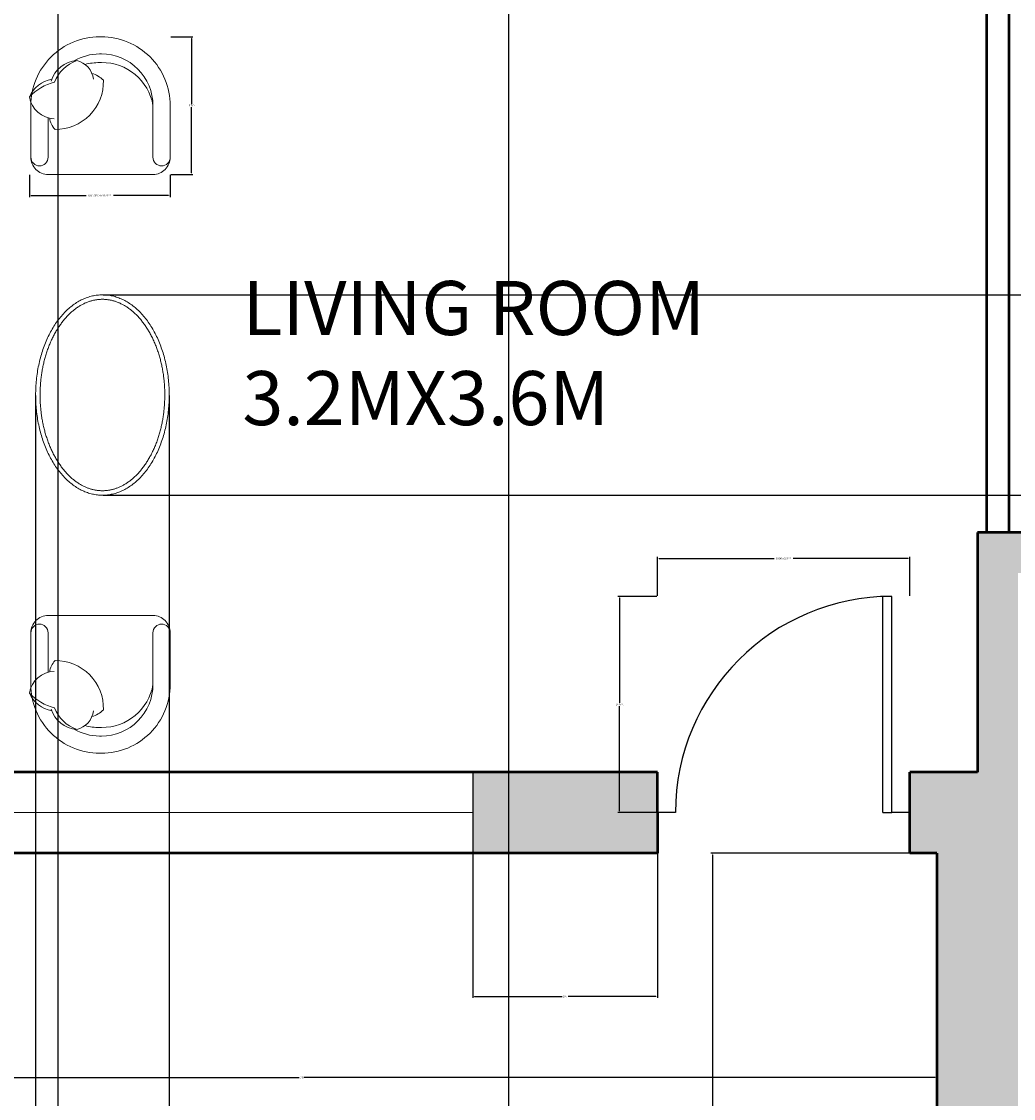
# Model space of a CAD drawing. Units: inches. Extents: x 3 to 380, y -485 to 60.
# Tile 3 of 8: x 67 to 177, y -390 to -270. Entities that reach past the tile are written whole.
import ezdxf

# ---------------------------------------------------------------- set-up
doc = ezdxf.new("R2010")
doc.units = ezdxf.units.IN
doc.header["$MEASUREMENT"] = 0
for name, color, linetype, lineweight in [('A-ANNO-DIMS', 2, 'Continuous', 18), ('A-AREA-IDEN', 7, 'Continuous', 25), ('A-DOOR', 3, 'Continuous', 25), ('A-FURN', 8, 'Continuous', 18), ('A-GLAZ', 4, 'Continuous', 18), ('A-WALL', 7, 'Continuous', 50), ('A-WALL-PATT', 252, 'Continuous', 13)]:
    doc.layers.add(name, color=color, linetype=linetype, lineweight=lineweight)
doc.styles.get("Standard").update_dxf_attribs({"font": 'arial.ttf'})
doc.dimstyles.get("Standard").update_dxf_attribs({"dimtxt": 0.18, "dimasz": 0.18, "dimexe": 0.18, "dimexo": 0.0625, "dimgap": 0.09, "dimtad": 0, "dimtih": 1, "dimtoh": 1, "dimdec": 0, "dimzin": 0, "dimdsep": 46, "dimlunit": 3, "dimtxsty": 'Standard', "dimcen": 0.09, "dimadec": 0, "dimazin": 0, "dimtfac": 1, "dimtdec": 0, "dimtofl": 0, "dimtmove": 0, "dimatfit": 3, "dimfxl": 1, "dimtolj": 1, "dimtzin": 0, "dimarcsym": 0})

# ---------------------------------------------------------------- blocks, each defined once
blk = doc.blocks.new('LOUNGE-CHAIR')
at = {"ltscale": 0.03}
blk.add_lwpolyline([(7.89, 0), (13.71, 0, 0.414214), (15.62, 1.91), (15.62, 7.64, 0.414214), (7.98, 15.28), (7.89, 15.28), (7.79, 15.28, 0.414214), (0.16, 7.64), (0.16, 1.91, 0.414214), (2.07, 0), (7.89, 0)], format="xyb", dxfattribs=at)
for points in [[(4.95, 12.61, -0.130591), (7.79, 13.37), (7.89, 13.37)], [(13.71, 7.64, 0.414214), (7.98, 13.37), (7.89, 13.37)], [(0, 8.6, -0.14773), (2.79, 10.24, -0.213343), (5.25, 12.65, -0.178662)], [(2.4, 10.37, -0.306663), (5.25, 12.65, -0.30633), (7.11, 10.57, 0.872847)], [(6.17, 12.21, -0.072384), (7.79, 12.41), (7.89, 12.41)], [(13.71, 7.64, 0.372719), (7.98, 12.41), (7.89, 12.41)], [(2.25, 6.25, 0.165541), (2.84, 4.99, 0.425989), (8.21, 10.46, 0.121523), (6.93, 11.21, -7.115464)], [(2.74, 6.19, -0.356772), (0, 8.6, -0.249542), (2.48, 10.58, 9.61688)], [(13.71, 7.64), (13.71, 1.91, 0.414214), (14.67, 0.95), (14.67, 0.95, 0.414214), (15.62, 1.91)], [(2.07, 6.3), (2.07, 1.91, -0.414214), (1.11, 0.95), (1.11, 0.95, -0.414214), (0.16, 1.91)]]:
    blk.add_lwpolyline(points, format="xyb")
blk = doc.blocks.new('WIN-60X9-SPLIT-JAMB')
for p, q in [((60, 9), (0, 9)), ((0, 9), (0, 0)), ((60, 4.5), (60, 9)), ((0, 4.5), (60, 4.5)), ((60, 4.5), (60, 0)), ((0, 0), (60, 0))]:
    blk.add_line(p, q)
blk = doc.blocks.new('DOOR-SWING-24')
for p, q in [((25, 0), (25, 24)), ((26, 0), (26, 24)), ((2, 0), (0, 0)), ((25, 0), (26, 0)), ((28, 0), (26, 0))]:
    blk.add_line(p, q)
blk.add_arc((26, 0), 24, 90, 180)
blk = doc.blocks.new('*D23')
at = {"layer": 'A-ANNO-DIMS', "color": 0, "lineweight": -2, "transparency": 16777216}
for p, q in [((137.84, -333.87), (137.84, -329.55)), ((138.02, -329.73), (150.79, -329.73)), ((165.66, -329.73), (152.89, -329.73)), ((165.84, -333.87), (165.84, -329.55))]:
    blk.add_line(p, q, dxfattribs=at)
at = {"layer": 'A-ANNO-DIMS', "color": 0, "transparency": 16777216}
for points in [[(138.02, -329.7), (138.02, -329.76), (137.84, -329.73)], [(165.66, -329.7), (165.66, -329.76), (165.84, -329.73)]]:
    blk.add_solid(points, dxfattribs=at)
at = {"layer": 'Defpoints', "color": 0, "transparency": 16777216}
for p in [(165.84, -329.73), (137.84, -333.93), (165.84, -333.93)]:
    blk.add_point(p, dxfattribs=at)
at = {"layer": 'A-ANNO-DIMS', "color": 0, "transparency": 16777216, "insert": (151.84, -329.73), "char_height": 0.18, "attachment_point": 5}
blk.add_mtext('\\A1;DOOR A 28 TYP.', dxfattribs=at)
blk = doc.blocks.new('*D24')
at = {"layer": 'A-ANNO-DIMS', "color": 0, "lineweight": -2, "transparency": 16777216}
for p, q in [((137.78, -333.93), (133.46, -333.93)), ((133.64, -334.11), (133.64, -345.75)), ((133.64, -357.75), (133.64, -346.11)), ((137.78, -357.93), (133.46, -357.93))]:
    blk.add_line(p, q, dxfattribs=at)
at = {"layer": 'A-ANNO-DIMS', "color": 0, "transparency": 16777216}
for points in [[(133.61, -334.11), (133.67, -334.11), (133.64, -333.93)], [(133.61, -357.75), (133.67, -357.75), (133.64, -357.93)]]:
    blk.add_solid(points, dxfattribs=at)
at = {"layer": 'Defpoints', "color": 0, "transparency": 16777216}
for p in [(133.64, -333.93), (137.84, -333.93), (137.84, -357.93)]:
    blk.add_point(p, dxfattribs=at)
at = {"layer": 'A-ANNO-DIMS', "color": 0, "transparency": 16777216, "insert": (133.64, -345.93), "char_height": 0.18, "attachment_point": 5}
blk.add_mtext('\\A1;24 TYP.', dxfattribs=at)
blk = doc.blocks.new('*D39')
at = {"layer": 'A-ANNO-DIMS', "color": 0, "lineweight": -2, "transparency": 16777216}
for p, q in [((68.15, -287.16), (68.15, -289.62)), ((83.78, -287.16), (83.78, -289.62)), ((68.33, -289.44), (74.45, -289.44)), ((83.6, -289.44), (77.48, -289.44))]:
    blk.add_line(p, q, dxfattribs=at)
at = {"layer": 'A-ANNO-DIMS', "color": 0, "transparency": 16777216}
for points in [[(68.33, -289.41), (68.33, -289.47), (68.15, -289.44)], [(83.6, -289.41), (83.6, -289.47), (83.78, -289.44)]]:
    blk.add_solid(points, dxfattribs=at)
at = {"layer": 'Defpoints', "color": 0, "transparency": 16777216}
for p in [(68.15, -287.1), (83.78, -287.1), (83.78, -289.44)]:
    blk.add_point(p, dxfattribs=at)
at = {"layer": 'A-ANNO-DIMS', "color": 0, "transparency": 16777216, "insert": (75.96, -289.44), "char_height": 0.18, "attachment_point": 5}
blk.add_mtext('\\A1;LOUNGE CHAIR 16 TYP.', dxfattribs=at)
blk = doc.blocks.new('*D40')
at = {"layer": 'A-ANNO-DIMS', "color": 0, "lineweight": -2, "transparency": 16777216}
for p, q in [((83.84, -271.82), (86.3, -271.82)), ((86.12, -272), (86.12, -279.28)), ((86.12, -286.92), (86.12, -279.64)), ((83.84, -287.1), (86.3, -287.1))]:
    blk.add_line(p, q, dxfattribs=at)
at = {"layer": 'A-ANNO-DIMS', "color": 0, "transparency": 16777216}
for points in [[(86.09, -272), (86.15, -272), (86.12, -271.82)], [(86.09, -286.92), (86.15, -286.92), (86.12, -287.1)]]:
    blk.add_solid(points, dxfattribs=at)
at = {"layer": 'Defpoints', "color": 0, "transparency": 16777216}
for p in [(83.78, -271.82), (86.12, -271.82), (83.78, -287.1)]:
    blk.add_point(p, dxfattribs=at)
at = {"layer": 'A-ANNO-DIMS', "color": 0, "transparency": 16777216, "insert": (86.12, -279.46), "char_height": 0.18, "attachment_point": 5}
blk.add_mtext('\\A1;15 TYP.', dxfattribs=at)
blk = doc.blocks.new('*D51')
at = {"layer": 'A-ANNO-DIMS', "color": 0, "lineweight": -2, "transparency": 16777216}
for p, q in [((151.9, 34.66), (379.92, 34.66)), ((379.74, 34.48), (379.74, -212.65)), ((379.74, -460.16), (379.74, -213.02)), ((354.9, -460.34), (379.92, -460.34))]:
    blk.add_line(p, q, dxfattribs=at)
at = {"layer": 'A-ANNO-DIMS', "color": 0, "transparency": 16777216}
for points in [[(379.71, 34.48), (379.77, 34.48), (379.74, 34.66)], [(379.71, -460.16), (379.77, -460.16), (379.74, -460.34)]]:
    blk.add_solid(points, dxfattribs=at)
at = {"layer": 'Defpoints', "color": 0, "transparency": 16777216}
for p in [(151.84, 34.66), (354.84, -460.34), (379.74, -460.34)]:
    blk.add_point(p, dxfattribs=at)
at = {"layer": 'A-ANNO-DIMS', "color": 0, "transparency": 16777216, "insert": (379.74, -212.84), "char_height": 0.18, "attachment_point": 5}
blk.add_mtext('\\A1;495', dxfattribs=at)
blk = doc.blocks.new('*D52')
at = {"layer": 'A-ANNO-DIMS', "color": 0, "lineweight": -2, "transparency": 16777216}
for p, q in [((27.84, -362.49), (27.84, -387.51)), ((168.84, -362.49), (168.84, -387.51)), ((28.02, -387.33), (98.08, -387.33)), ((168.66, -387.33), (98.6, -387.33))]:
    blk.add_line(p, q, dxfattribs=at)
at = {"layer": 'A-ANNO-DIMS', "color": 0, "transparency": 16777216}
for points in [[(28.02, -387.3), (28.02, -387.36), (27.84, -387.33)], [(168.66, -387.3), (168.66, -387.36), (168.84, -387.33)]]:
    blk.add_solid(points, dxfattribs=at)
at = {"layer": 'Defpoints', "color": 0, "transparency": 16777216}
for p in [(27.84, -362.43), (168.84, -362.43), (27.84, -387.33)]:
    blk.add_point(p, dxfattribs=at)
at = {"layer": 'A-ANNO-DIMS', "color": 0, "transparency": 16777216, "insert": (98.34, -387.33), "char_height": 0.18, "attachment_point": 5}
blk.add_mtext('\\A1;141', dxfattribs=at)
blk = doc.blocks.new('*D56')
at = {"layer": 'A-ANNO-DIMS', "color": 0, "lineweight": -2, "transparency": 16777216}
for p, q in [((168.78, -362.43), (143.76, -362.43)), ((143.94, -362.61), (143.94, -411.2)), ((143.94, -460.16), (143.94, -411.56)), ((168.78, -460.34), (143.76, -460.34))]:
    blk.add_line(p, q, dxfattribs=at)
at = {"layer": 'A-ANNO-DIMS', "color": 0, "transparency": 16777216}
for points in [[(143.91, -362.61), (143.97, -362.61), (143.94, -362.43)], [(143.91, -460.16), (143.97, -460.16), (143.94, -460.34)]]:
    blk.add_solid(points, dxfattribs=at)
at = {"layer": 'Defpoints', "color": 0, "transparency": 16777216}
for p in [(143.94, -362.43), (168.84, -362.43), (168.84, -460.34)]:
    blk.add_point(p, dxfattribs=at)
at = {"layer": 'A-ANNO-DIMS', "color": 0, "transparency": 16777216, "insert": (143.94, -411.38), "char_height": 0.18, "attachment_point": 5}
blk.add_mtext('\\A1;97.9', dxfattribs=at)
blk = doc.blocks.new('*D82')
at = {"layer": 'A-ANNO-DIMS', "color": 0, "lineweight": -2, "transparency": 16777216}
for p, q in [((117.34, -353.49), (117.34, -378.51)), ((137.84, -353.49), (137.84, -378.51)), ((117.52, -378.33), (127.26, -378.33)), ((137.66, -378.33), (127.92, -378.33))]:
    blk.add_line(p, q, dxfattribs=at)
at = {"layer": 'A-ANNO-DIMS', "color": 0, "transparency": 16777216}
for points in [[(117.52, -378.3), (117.52, -378.36), (117.34, -378.33)], [(137.66, -378.3), (137.66, -378.36), (137.84, -378.33)]]:
    blk.add_solid(points, dxfattribs=at)
at = {"layer": 'Defpoints', "color": 0, "transparency": 16777216}
for p in [(117.34, -353.43), (137.84, -353.43), (117.34, -378.33)]:
    blk.add_point(p, dxfattribs=at)
at = {"layer": 'A-ANNO-DIMS', "color": 0, "transparency": 16777216, "insert": (127.59, -378.33), "char_height": 0.18, "attachment_point": 5}
blk.add_mtext('\\A1;20.5', dxfattribs=at)
blk = doc.blocks.new('*D93')
at = {"layer": 'A-ANNO-DIMS', "color": 0, "lineweight": -2, "transparency": 16777216}
for p, q in [((71.32, -23.85), (71.32, -485.42)), ((121.32, -23.85), (121.32, -485.42)), ((71.5, -485.24), (95.92, -485.24)), ((121.14, -485.24), (96.72, -485.24))]:
    blk.add_line(p, q, dxfattribs=at)
at = {"layer": 'A-ANNO-DIMS', "color": 0, "transparency": 16777216}
for points in [[(71.5, -485.21), (71.5, -485.27), (71.32, -485.24)], [(121.14, -485.21), (121.14, -485.27), (121.32, -485.24)]]:
    blk.add_solid(points, dxfattribs=at)
at = {"layer": 'Defpoints', "color": 0, "transparency": 16777216}
for p in [(71.32, -23.79), (121.32, -23.79), (71.32, -485.24)]:
    blk.add_point(p, dxfattribs=at)
at = {"layer": 'A-ANNO-DIMS', "color": 0, "transparency": 16777216, "insert": (96.32, -485.24), "char_height": 0.18, "attachment_point": 5}
blk.add_mtext('\\A1;49.99', dxfattribs=at)
blk = doc.blocks.new('*D99')
at = {"layer": 'A-ANNO-DIMS', "color": 0, "lineweight": -2, "transparency": 16777216}
for p, q in [((76.32, -300.46), (379.92, -300.46)), ((379.74, -300.64), (379.74, -311.4)), ((379.74, -322.52), (379.74, -311.76)), ((76.32, -322.7), (379.92, -322.7))]:
    blk.add_line(p, q, dxfattribs=at)
at = {"layer": 'A-ANNO-DIMS', "color": 0, "transparency": 16777216}
for points in [[(379.71, -300.64), (379.77, -300.64), (379.74, -300.46)], [(379.71, -322.52), (379.77, -322.52), (379.74, -322.7)]]:
    blk.add_solid(points, dxfattribs=at)
at = {"layer": 'Defpoints', "color": 0, "transparency": 16777216}
for p in [(76.25, -300.46), (76.25, -322.7), (379.74, -322.7)]:
    blk.add_point(p, dxfattribs=at)
at = {"layer": 'A-ANNO-DIMS', "color": 0, "transparency": 16777216, "insert": (379.74, -311.58), "char_height": 0.18, "attachment_point": 5}
blk.add_mtext('\\A1;22.236', dxfattribs=at)
blk = doc.blocks.new('*D100')
at = {"layer": 'A-ANNO-DIMS', "color": 0, "lineweight": -2, "transparency": 16777216}
for p, q in [((68.84, -311.64), (68.84, -485.42)), ((83.67, -311.64), (83.67, -485.42)), ((69.02, -485.24), (75.8, -485.24)), ((83.49, -485.24), (76.71, -485.24))]:
    blk.add_line(p, q, dxfattribs=at)
at = {"layer": 'A-ANNO-DIMS', "color": 0, "transparency": 16777216}
for points in [[(69.02, -485.21), (69.02, -485.27), (68.84, -485.24)], [(83.49, -485.21), (83.49, -485.27), (83.67, -485.24)]]:
    blk.add_solid(points, dxfattribs=at)
at = {"layer": 'Defpoints', "color": 0, "transparency": 16777216}
for p in [(68.84, -311.58), (83.67, -311.58), (83.67, -485.24)]:
    blk.add_point(p, dxfattribs=at)
at = {"layer": 'A-ANNO-DIMS', "color": 0, "transparency": 16777216, "insert": (76.25, -485.24), "char_height": 0.18, "attachment_point": 5}
blk.add_mtext('\\A1;14.824', dxfattribs=at)

msp = doc.modelspace()

# ---------------------------------------------------------------- hatches: boundary and pattern name
at = {"layer": 'A-WALL-PATT'}
h = msp.add_hatch(color=256, dxfattribs=at)
h.dxf.hatch_style = 1
h.paths.add_polyline_path([(36.8404, 6.1643), (51.3404, 6.1643), (51.3404, 15.1643), (27.8404, 15.1643), (27.8404, -143.6318), (36.8404, -143.6318)])
h.paths.add_polyline_path([(125.8404, 10.6643), (125.8404, 15.1643), (111.3404, 15.1643), (111.3404, 6.1643), (125.8404, 6.1643)])
h.paths.add_polyline_path([(170.6358, 15.1643), (153.8404, 15.1643), (153.8404, 6.1643), (156.8404, 6.1643), (156.8404, -82.3357), (173.3404, -82.3357), (173.3404, -130.3357), (177.8404, -130.3357), (180.8404, -130.3357), (180.8404, -125.8357), (177.8404, -125.8357), (177.8404, -82.3357), (201.8404, -82.3357), (201.8404, -38.0857), (197.3404, -38.0857), (197.3404, -77.8357), (161.3404, -77.8357), (161.3404, 6.1643), (170.6358, 6.1643)])
h.paths.add_polyline_path([(241.3739, 15.1643), (194.6358, 15.1643), (194.6358, 6.1643), (241.3739, 6.1643)])
h.paths.add_polyline_path([(201.8404, 6.1643), (197.3404, 6.1643), (197.3404, -12.1977), (201.8404, -12.1977)], flags=17)
h.paths.add_polyline_path([(354.8404, 15.1643), (301.3739, 15.1643), (301.3739, 6.1643), (345.8404, 6.1643), (345.8404, -34.0336), (354.8404, -34.0336)])
h.paths.add_polyline_path([(354.8404, -94.0336), (345.8404, -94.0336), (345.8404, -159.3738), (354.8404, -159.3738)])
h.paths.add_polyline_path([(345.8404, -125.8357), (209.3404, -125.8357), (209.3404, -205.8357), (211.5904, -205.8357), (213.8404, -205.8357), (213.8404, -130.3357), (345.8404, -130.3357)])
h.paths.add_polyline_path([(36.8404, -203.6318), (27.8404, -203.6318), (27.8404, -270.1269), (36.8404, -270.1269)])
h.paths.add_polyline_path([(36.8404, -330.1269), (27.8404, -330.1269), (27.8404, -362.428), (57.3404, -362.428), (57.3404, -353.428), (36.8404, -353.428)])
h.paths.add_polyline_path([(177.8404, -331.3357), (180.8404, -331.3357), (180.8404, -326.8357), (173.3404, -326.8357), (173.3404, -353.428), (165.8404, -353.428), (165.8404, -362.428), (168.8404, -362.428), (168.8404, -451.3357), (168.8404, -460.3357), (231.8404, -460.3357), (231.8404, -451.3357), (177.8404, -451.3357)])
h.paths.add_polyline_path([(354.8404, -305.1003), (345.8404, -305.1003), (345.8404, -363.2829), (354.8404, -363.2829)])
h.paths.add_polyline_path([(345.8404, -326.8357), (213.8404, -326.8357), (213.8404, -312.8357), (211.5904, -312.8357), (209.3404, -312.8357), (209.3404, -331.3357), (345.8404, -331.3357)])
h.paths.add_polyline_path([(345.8404, -262.3357), (237.8404, -262.3357), (237.8404, -233.8357), (209.3404, -233.8357), (209.3404, -284.8357), (213.8404, -284.8357), (213.8404, -238.3357), (233.3404, -238.3357), (233.3404, -266.8357), (345.8404, -266.8357)])
h.paths.add_polyline_path([(354.8404, -219.3738), (345.8404, -219.3738), (345.8404, -281.1003), (354.8404, -281.1003)])
h = msp.add_hatch(color=256, dxfattribs=at)
h.dxf.hatch_style = 1
h.paths.add_polyline_path([(137.8404, -353.428), (117.3404, -353.428), (117.3404, -357.928), (117.3404, -362.428), (137.8404, -362.428), (137.8404, -357.928)])

# ---------------------------------------------------------------- linework, layer by layer
at = {"layer": 'A-FURN', "ltscale": 0.03}
msp.add_polyline3d([(76.2547, -300.4625, 0), (76.1145, -300.4645, 0), (75.9742, -300.4705, 0), (75.8341, -300.4804, 0), (75.6942, -300.4943, 0), (75.5544, -300.5122, 0), (75.4149, -300.5341, 0), (75.2757, -300.5599, 0), (75.1368, -300.5897, 0), (74.9983, -300.6234, 0), (74.8603, -300.661, 0), (74.7228, -300.7026, 0), (74.5859, -300.748, 0), (74.4495, -300.7973, 0), (74.3138, -300.8505, 0), (74.1787, -300.9075, 0), (74.0445, -300.9683, 0), (73.911, -301.033, 0), (73.7783, -301.1014, 0), (73.6466, -301.1736, 0), (73.5157, -301.2495, 0), (73.3859, -301.3291, 0), (73.2571, -301.4123, 0), (73.1293, -301.4992, 0), (73.0027, -301.5898, 0), (72.8772, -301.6839, 0), (72.753, -301.7815, 0), (72.63, -301.8827, 0), (72.5083, -301.9873, 0), (72.3879, -302.0954, 0), (72.269, -302.2068, 0), (72.1514, -302.3216, 0), (72.0353, -302.4398, 0), (71.9208, -302.5612, 0), (71.8078, -302.6858, 0), (71.6963, -302.8137, 0), (71.5865, -302.9446, 0), (71.4784, -303.0787, 0), (71.372, -303.2158, 0), (71.2674, -303.3559, 0), (71.1645, -303.4989, 0), (71.0635, -303.6449, 0), (70.9643, -303.7936, 0), (70.867, -303.9452, 0), (70.7716, -304.0995, 0), (70.6782, -304.2565, 0), (70.5868, -304.4161, 0), (70.4974, -304.5783, 0), (70.4101, -304.743, 0), (70.3249, -304.9101, 0), (70.2418, -305.0796, 0), (70.1609, -305.2515, 0), (70.0821, -305.4256, 0), (70.0056, -305.6019, 0), (69.9313, -305.7804, 0), (69.8592, -305.9609, 0), (69.7895, -306.1434, 0), (69.722, -306.3279, 0), (69.6569, -306.5143, 0), (69.5942, -306.7025, 0), (69.5339, -306.8925, 0), (69.4759, -307.0841, 0), (69.4204, -307.2773, 0), (69.3673, -307.4721, 0), (69.3167, -307.6683, 0), (69.2686, -307.866, 0), (69.223, -308.0649, 0), (69.1799, -308.2652, 0), (69.1393, -308.4666, 0), (69.1013, -308.6691, 0), (69.0659, -308.8727, 0), (69.033, -309.0773, 0), (69.0027, -309.2827, 0), (68.975, -309.489, 0), (68.9499, -309.696, 0), (68.9275, -309.9037, 0), (68.9076, -310.112, 0), (68.8904, -310.3208, 0), (68.8759, -310.5301, 0), (68.8639, -310.7397, 0), (68.8546, -310.9496, 0), (68.848, -311.1598, 0), (68.844, -311.3701, 0), (68.8427, -311.5805, 0), (68.844, -311.7909, 0), (68.848, -312.0013, 0), (68.8546, -312.2114, 0), (68.8639, -312.4214, 0), (68.8759, -312.631, 0), (68.8904, -312.8403, 0), (68.9076, -313.0491, 0), (68.9275, -313.2574, 0), (68.9499, -313.4651, 0), (68.975, -313.6721, 0), (69.0027, -313.8784, 0), (69.033, -314.0838, 0), (69.0659, -314.2884, 0), (69.1013, -314.492, 0), (69.1393, -314.6945, 0), (69.1799, -314.8959, 0), (69.223, -315.0962, 0), (69.2686, -315.2951, 0), (69.3167, -315.4928, 0), (69.3673, -315.689, 0), (69.4204, -315.8838, 0), (69.4759, -316.077, 0), (69.5339, -316.2686, 0), (69.5942, -316.4586, 0), (69.6569, -316.6468, 0), (69.722, -316.8331, 0), (69.7895, -317.0176, 0), (69.8592, -317.2002, 0), (69.9313, -317.3807, 0), (70.0056, -317.5592, 0), (70.0821, -317.7355, 0), (70.1609, -317.9096, 0), (70.2418, -318.0815, 0), (70.3249, -318.251, 0), (70.4101, -318.4181, 0), (70.4974, -318.5828, 0), (70.5868, -318.745, 0), (70.6782, -318.9046, 0), (70.7716, -319.0616, 0), (70.867, -319.2159, 0), (70.9643, -319.3674, 0), (71.0635, -319.5162, 0), (71.1645, -319.6622, 0), (71.2674, -319.8052, 0), (71.372, -319.9453, 0), (71.4784, -320.0824, 0), (71.5865, -320.2165, 0), (71.6963, -320.3474, 0), (71.8078, -320.4753, 0), (71.9208, -320.5999, 0), (72.0353, -320.7213, 0), (72.1514, -320.8394, 0), (72.269, -320.9543, 0), (72.3879, -321.0657, 0), (72.5083, -321.1738, 0), (72.63, -321.2784, 0), (72.753, -321.3796, 0), (72.8772, -321.4772, 0), (73.0027, -321.5713, 0), (73.1293, -321.6618, 0), (73.2571, -321.7488, 0), (73.3859, -321.832, 0), (73.5157, -321.9116, 0), (73.6466, -321.9875, 0), (73.7783, -322.0597, 0), (73.911, -322.1281, 0), (74.0445, -322.1928, 0), (74.1787, -322.2536, 0), (74.3138, -322.3106, 0), (74.4495, -322.3638, 0), (74.5859, -322.4131, 0), (74.7228, -322.4585, 0), (74.8603, -322.5001, 0), (74.9983, -322.5377, 0), (75.1368, -322.5714, 0), (75.2757, -322.6012, 0), (75.4149, -322.627, 0), (75.5544, -322.6488, 0), (75.6942, -322.6667, 0), (75.8341, -322.6807, 0), (75.9742, -322.6906, 0), (76.1145, -322.6966, 0), (76.2547, -322.6986, 0), (76.395, -322.6966, 0), (76.5352, -322.6906, 0), (76.6753, -322.6807, 0), (76.8153, -322.6667, 0), (76.955, -322.6488, 0), (77.0946, -322.627, 0), (77.2338, -322.6012, 0), (77.3726, -322.5714, 0), (77.5111, -322.5377, 0), (77.6491, -322.5001, 0), (77.7866, -322.4585, 0), (77.9236, -322.4131, 0), (78.0599, -322.3638, 0), (78.1957, -322.3106, 0), (78.3307, -322.2536, 0), (78.465, -322.1928, 0), (78.5985, -322.1281, 0), (78.7311, -322.0597, 0), (78.8629, -321.9875, 0), (78.9937, -321.9116, 0), (79.1235, -321.832, 0), (79.2524, -321.7488, 0), (79.3801, -321.6618, 0), (79.5067, -321.5713, 0), (79.6322, -321.4772, 0), (79.7565, -321.3796, 0), (79.8795, -321.2784, 0), (80.0012, -321.1738, 0), (80.1215, -321.0657, 0), (80.2405, -320.9543, 0), (80.358, -320.8394, 0), (80.4741, -320.7213, 0), (80.5887, -320.5999, 0), (80.7017, -320.4753, 0), (80.8131, -320.3474, 0), (80.9229, -320.2165, 0), (81.031, -320.0824, 0), (81.1374, -319.9453, 0), (81.2421, -319.8052, 0), (81.3449, -319.6622, 0), (81.446, -319.5162, 0), (81.5452, -319.3674, 0), (81.6425, -319.2159, 0), (81.7378, -319.0616, 0), (81.8312, -318.9046, 0), (81.9226, -318.745, 0), (82.012, -318.5828, 0), (82.0993, -318.4181, 0), (82.1845, -318.251, 0), (82.2676, -318.0815, 0), (82.3486, -317.9096, 0), (82.4273, -317.7355, 0), (82.5039, -317.5592, 0), (82.5782, -317.3807, 0), (82.6502, -317.2002, 0), (82.72, -317.0176, 0), (82.7874, -316.8331, 0), (82.8525, -316.6468, 0), (82.9152, -316.4586, 0), (82.9756, -316.2686, 0), (83.0335, -316.077, 0), (83.089, -315.8838, 0), (83.1421, -315.689, 0), (83.1927, -315.4928, 0), (83.2408, -315.2951, 0), (83.2864, -315.0962, 0), (83.3295, -314.8959, 0), (83.3701, -314.6945, 0), (83.4081, -314.492, 0), (83.4436, -314.2884, 0), (83.4764, -314.0838, 0), (83.5067, -313.8784, 0), (83.5344, -313.6721, 0), (83.5595, -313.4651, 0), (83.582, -313.2574, 0), (83.6018, -313.0491, 0), (83.619, -312.8403, 0), (83.6336, -312.631, 0), (83.6455, -312.4214, 0), (83.6548, -312.2114, 0), (83.6614, -312.0013, 0), (83.6654, -311.7909, 0), (83.6667, -311.5805, 0), (83.6654, -311.3701, 0), (83.6614, -311.1598, 0), (83.6548, -310.9496, 0), (83.6455, -310.7397, 0), (83.6336, -310.5301, 0), (83.619, -310.3208, 0), (83.6018, -310.112, 0), (83.582, -309.9037, 0), (83.5595, -309.696, 0), (83.5344, -309.489, 0), (83.5067, -309.2827, 0), (83.4764, -309.0773, 0), (83.4436, -308.8727, 0), (83.4081, -308.6691, 0), (83.3701, -308.4666, 0), (83.3295, -308.2652, 0), (83.2864, -308.0649, 0), (83.2408, -307.866, 0), (83.1927, -307.6683, 0), (83.1421, -307.4721, 0), (83.089, -307.2773, 0), (83.0335, -307.0841, 0), (82.9756, -306.8925, 0), (82.9152, -306.7025, 0), (82.8525, -306.5143, 0), (82.7874, -306.3279, 0), (82.72, -306.1434, 0), (82.6502, -305.9609, 0), (82.5782, -305.7804, 0), (82.5039, -305.6019, 0), (82.4273, -305.4256, 0), (82.3486, -305.2515, 0), (82.2676, -305.0796, 0), (82.1845, -304.9101, 0), (82.0993, -304.743, 0), (82.012, -304.5783, 0), (81.9226, -304.4161, 0), (81.8312, -304.2565, 0), (81.7378, -304.0995, 0), (81.6425, -303.9452, 0), (81.5452, -303.7936, 0), (81.446, -303.6449, 0), (81.3449, -303.4989, 0), (81.2421, -303.3559, 0), (81.1374, -303.2158, 0), (81.031, -303.0787, 0), (80.9229, -302.9446, 0), (80.8131, -302.8137, 0), (80.7017, -302.6858, 0), (80.5887, -302.5612, 0), (80.4741, -302.4398, 0), (80.358, -302.3216, 0), (80.2405, -302.2068, 0), (80.1215, -302.0954, 0), (80.0012, -301.9873, 0), (79.8795, -301.8827, 0), (79.7565, -301.7815, 0), (79.6322, -301.6839, 0), (79.5067, -301.5898, 0), (79.3801, -301.4992, 0), (79.2524, -301.4123, 0), (79.1235, -301.3291, 0), (78.9937, -301.2495, 0), (78.8629, -301.1736, 0), (78.7311, -301.1014, 0), (78.5985, -301.033, 0), (78.465, -300.9683, 0), (78.3307, -300.9075, 0), (78.1957, -300.8505, 0), (78.0599, -300.7973, 0), (77.9236, -300.748, 0), (77.7866, -300.7026, 0), (77.6491, -300.661, 0), (77.5111, -300.6234, 0), (77.3726, -300.5897, 0), (77.2338, -300.5599, 0), (77.0946, -300.5341, 0), (76.955, -300.5122, 0), (76.8153, -300.4943, 0), (76.6753, -300.4804, 0), (76.5352, -300.4705, 0), (76.395, -300.4645, 0), (76.2547, -300.4625, 0)], dxfattribs=at)
at = {"layer": 'A-FURN'}
msp.add_polyline3d([(76.2547, -300.9566, 0), (76.1789, -300.9573, 0), (76.1028, -300.9592, 0), (76.0263, -300.9625, 0), (75.9495, -300.9671, 0), (75.8723, -300.9731, 0), (75.7949, -300.9805, 0), (75.7171, -300.9892, 0), (75.6391, -300.9994, 0), (75.5608, -301.0109, 0), (75.4822, -301.024, 0), (75.4034, -301.0384, 0), (75.3243, -301.0544, 0), (75.245, -301.0719, 0), (75.1655, -301.0908, 0), (75.0858, -301.1113, 0), (75.0058, -301.1334, 0), (74.9257, -301.157, 0), (74.8454, -301.1822, 0), (74.7649, -301.2089, 0), (74.6843, -301.2373, 0), (74.6035, -301.2674, 0), (74.5226, -301.2991, 0), (74.4415, -301.3325, 0), (74.3605, -301.3675, 0), (74.2793, -301.4042, 0), (74.1981, -301.4427, 0), (74.117, -301.4828, 0), (74.0358, -301.5246, 0), (73.9547, -301.5681, 0), (73.8737, -301.6132, 0), (73.7927, -301.6601, 0), (73.7119, -301.7087, 0), (73.6312, -301.759, 0), (73.5507, -301.811, 0), (73.4704, -301.8647, 0), (73.3902, -301.9201, 0), (73.3104, -301.9772, 0), (73.2307, -302.036, 0), (73.1514, -302.0965, 0), (73.0724, -302.1588, 0), (72.9937, -302.2228, 0), (72.9154, -302.2885, 0), (72.8374, -302.3561, 0), (72.7599, -302.4255, 0), (72.6827, -302.4967, 0), (72.606, -302.5697, 0), (72.5298, -302.6445, 0), (72.454, -302.721, 0), (72.3787, -302.7993, 0), (72.304, -302.8792, 0), (72.2298, -302.9608, 0), (72.1561, -303.044, 0), (72.083, -303.1289, 0), (72.0105, -303.2153, 0), (71.9387, -303.3033, 0), (71.8674, -303.3929, 0), (71.7969, -303.4839, 0), (71.727, -303.5764, 0), (71.6578, -303.6704, 0), (71.5893, -303.7658, 0), (71.5216, -303.8627, 0), (71.4546, -303.9609, 0), (71.3885, -304.0604, 0), (71.3231, -304.1613, 0), (71.2585, -304.2635, 0), (71.1948, -304.367, 0), (71.1319, -304.4717, 0), (71.0699, -304.5776, 0), (71.0089, -304.6847, 0), (70.9487, -304.7931, 0), (70.8895, -304.9025, 0), (70.8313, -305.0131, 0), (70.774, -305.1248, 0), (70.7178, -305.2375, 0), (70.6625, -305.3513, 0), (70.6083, -305.4661, 0), (70.5552, -305.5819, 0), (70.5032, -305.6987, 0), (70.4522, -305.8164, 0), (70.4024, -305.935, 0), (70.3538, -306.0545, 0), (70.3063, -306.1749, 0), (70.26, -306.2961, 0), (70.2149, -306.4179, 0), (70.1709, -306.5402, 0), (70.1282, -306.6627, 0), (70.0867, -306.7856, 0), (70.0463, -306.9088, 0), (70.0072, -307.0323, 0), (69.9691, -307.1561, 0), (69.9323, -307.2801, 0), (69.8966, -307.4045, 0), (69.8621, -307.5292, 0), (69.8287, -307.6541, 0), (69.7965, -307.7792, 0), (69.7654, -307.9047, 0), (69.7355, -308.0303, 0), (69.7066, -308.1562, 0), (69.6789, -308.2823, 0), (69.6524, -308.4087, 0), (69.6269, -308.5352, 0), (69.6025, -308.662, 0), (69.5793, -308.7889, 0), (69.5571, -308.916, 0), (69.5361, -309.0433, 0), (69.5161, -309.1708, 0), (69.4972, -309.2984, 0), (69.4794, -309.4261, 0), (69.4627, -309.554, 0), (69.447, -309.6821, 0), (69.4324, -309.8102, 0), (69.4189, -309.9385, 0), (69.4064, -310.0669, 0), (69.395, -310.1954, 0), (69.3846, -310.324, 0), (69.3752, -310.4526, 0), (69.3669, -310.5813, 0), (69.3596, -310.7101, 0), (69.3533, -310.839, 0), (69.3481, -310.9679, 0), (69.3438, -311.0968, 0), (69.3406, -311.2258, 0), (69.3383, -311.3548, 0), (69.3371, -311.4838, 0), (69.3369, -311.6128, 0), (69.3376, -311.7418, 0), (69.3393, -311.8708, 0), (69.3421, -311.9998, 0), (69.3458, -312.1287, 0), (69.3506, -312.2577, 0), (69.3563, -312.3865, 0), (69.3631, -312.5154, 0), (69.3709, -312.6441, 0), (69.3798, -312.7728, 0), (69.3896, -312.9014, 0), (69.4006, -313.03, 0), (69.4125, -313.1584, 0), (69.4255, -313.2867, 0), (69.4396, -313.4149, 0), (69.4547, -313.543, 0), (69.4709, -313.671, 0), (69.4882, -313.7988, 0), (69.5065, -313.9265, 0), (69.526, -314.0541, 0), (69.5465, -314.1814, 0), (69.5681, -314.3087, 0), (69.5908, -314.4357, 0), (69.6146, -314.5625, 0), (69.6395, -314.6892, 0), (69.6655, -314.8156, 0), (69.6926, -314.9418, 0), (69.7209, -315.0678, 0), (69.7503, -315.1936, 0), (69.7808, -315.3192, 0), (69.8125, -315.4445, 0), (69.8453, -315.5695, 0), (69.8792, -315.6943, 0), (69.9143, -315.8188, 0), (69.9506, -315.943, 0), (69.988, -316.067, 0), (70.0266, -316.1906, 0), (70.0664, -316.314, 0), (70.1073, -316.437, 0), (70.1494, -316.5597, 0), (70.1927, -316.6821, 0), (70.2373, -316.8041, 0), (70.283, -316.9257, 0), (70.3299, -317.0465, 0), (70.378, -317.1665, 0), (70.4272, -317.2855, 0), (70.4776, -317.4037, 0), (70.5291, -317.5209, 0), (70.5816, -317.6372, 0), (70.6353, -317.7525, 0), (70.69, -317.8668, 0), (70.7458, -317.9801, 0), (70.8025, -318.0923, 0), (70.8603, -318.2034, 0), (70.919, -318.3134, 0), (70.9787, -318.4223, 0), (71.0393, -318.5301, 0), (71.1008, -318.6366, 0), (71.1632, -318.7419, 0), (71.2265, -318.846, 0), (71.2907, -318.9489, 0), (71.3557, -319.0504, 0), (71.4214, -319.1506, 0), (71.488, -319.2495, 0), (71.5554, -319.347, 0), (71.6235, -319.4431, 0), (71.6923, -319.5378, 0), (71.7618, -319.6311, 0), (71.8321, -319.7229, 0), (71.903, -319.8132, 0), (71.9745, -319.9019, 0), (72.0467, -319.9892, 0), (72.1195, -320.0748, 0), (72.1929, -320.1589, 0), (72.2668, -320.2413, 0), (72.3413, -320.3221, 0), (72.4163, -320.4012, 0), (72.4918, -320.4785, 0), (72.5678, -320.5542, 0), (72.6443, -320.6281, 0), (72.7212, -320.7002, 0), (72.7986, -320.7706, 0), (72.8764, -320.839, 0), (72.9545, -320.9057, 0), (73.033, -320.9705, 0), (73.1119, -321.0336, 0), (73.191, -321.095, 0), (73.2705, -321.1547, 0), (73.3503, -321.2127, 0), (73.4303, -321.2689, 0), (73.5105, -321.3235, 0), (73.5909, -321.3763, 0), (73.6715, -321.4275, 0), (73.7523, -321.4769, 0), (73.8332, -321.5246, 0), (73.9142, -321.5707, 0), (73.9953, -321.615, 0), (74.0764, -321.6576, 0), (74.1576, -321.6986, 0), (74.2387, -321.7378, 0), (74.3199, -321.7754, 0), (74.401, -321.8113, 0), (74.4821, -321.8455, 0), (74.563, -321.8781, 0), (74.6439, -321.9089, 0), (74.7246, -321.9382, 0), (74.8052, -321.9657, 0), (74.8855, -321.9917, 0), (74.9658, -322.0161, 0), (75.0458, -322.0389, 0), (75.1256, -322.0602, 0), (75.2053, -322.0799, 0), (75.2847, -322.0982, 0), (75.3639, -322.1149, 0), (75.4428, -322.1301, 0), (75.5215, -322.1438, 0), (75.6, -322.1561, 0), (75.6781, -322.167, 0), (75.756, -322.1764, 0), (75.8336, -322.1845, 0), (75.9109, -322.1911, 0), (75.9879, -322.1964, 0), (76.0646, -322.2004, 0), (76.1409, -322.203, 0), (76.2169, -322.2043, 0), (76.2926, -322.2043, 0), (76.3686, -322.203, 0), (76.4449, -322.2004, 0), (76.5215, -322.1964, 0), (76.5985, -322.1911, 0), (76.6758, -322.1845, 0), (76.7534, -322.1764, 0), (76.8313, -322.167, 0), (76.9095, -322.1561, 0), (76.9879, -322.1438, 0), (77.0666, -322.1301, 0), (77.1456, -322.1149, 0), (77.2247, -322.0982, 0), (77.3042, -322.0799, 0), (77.3838, -322.0602, 0), (77.4636, -322.0389, 0), (77.5437, -322.0161, 0), (77.6239, -321.9917, 0), (77.7043, -321.9657, 0), (77.7848, -321.9382, 0), (77.8656, -321.9089, 0), (77.9464, -321.8781, 0), (78.0274, -321.8455, 0), (78.1084, -321.8113, 0), (78.1896, -321.7754, 0), (78.2707, -321.7378, 0), (78.3519, -321.6986, 0), (78.433, -321.6576, 0), (78.5142, -321.615, 0), (78.5953, -321.5707, 0), (78.6762, -321.5246, 0), (78.7571, -321.4769, 0), (78.8379, -321.4275, 0), (78.9185, -321.3763, 0), (78.9989, -321.3235, 0), (79.0792, -321.2689, 0), (79.1592, -321.2127, 0), (79.2389, -321.1547, 0), (79.3184, -321.095, 0), (79.3976, -321.0336, 0), (79.4764, -320.9705, 0), (79.5549, -320.9057, 0), (79.6331, -320.839, 0), (79.7108, -320.7706, 0), (79.7882, -320.7002, 0), (79.8651, -320.6281, 0), (79.9416, -320.5542, 0), (80.0176, -320.4785, 0), (80.0931, -320.4012, 0), (80.1682, -320.3221, 0), (80.2426, -320.2413, 0), (80.3166, -320.1589, 0), (80.39, -320.0748, 0), (80.4627, -319.9892, 0), (80.5349, -319.9019, 0), (80.6065, -319.8132, 0), (80.6774, -319.7229, 0), (80.7476, -319.6311, 0), (80.8171, -319.5378, 0), (80.886, -319.4431, 0), (80.9541, -319.347, 0), (81.0214, -319.2495, 0), (81.088, -319.1506, 0), (81.1538, -319.0504, 0), (81.2188, -318.9489, 0), (81.2829, -318.846, 0), (81.3462, -318.7419, 0), (81.4086, -318.6366, 0), (81.4701, -318.5301, 0), (81.5308, -318.4223, 0), (81.5904, -318.3134, 0), (81.6492, -318.2034, 0), (81.7069, -318.0923, 0), (81.7637, -317.9801, 0), (81.8194, -317.8668, 0), (81.8741, -317.7525, 0), (81.9278, -317.6372, 0), (81.9804, -317.5209, 0), (82.0319, -317.4037, 0), (82.0822, -317.2855, 0), (82.1315, -317.1665, 0), (82.1796, -317.0465, 0), (82.2265, -316.9257, 0), (82.2722, -316.8041, 0), (82.3167, -316.6821, 0), (82.36, -316.5597, 0), (82.4021, -316.437, 0), (82.4431, -316.314, 0), (82.4828, -316.1906, 0), (82.5214, -316.067, 0), (82.5589, -315.943, 0), (82.5951, -315.8188, 0), (82.6302, -315.6943, 0), (82.6642, -315.5695, 0), (82.697, -315.4445, 0), (82.7286, -315.3192, 0), (82.7591, -315.1936, 0), (82.7885, -315.0678, 0), (82.8168, -314.9418, 0), (82.8439, -314.8156, 0), (82.8699, -314.6892, 0), (82.8949, -314.5625, 0), (82.9187, -314.4357, 0), (82.9414, -314.3087, 0), (82.963, -314.1814, 0), (82.9835, -314.0541, 0), (83.0029, -313.9265, 0), (83.0212, -313.7988, 0), (83.0385, -313.671, 0), (83.0547, -313.543, 0), (83.0698, -313.4149, 0), (83.0839, -313.2867, 0), (83.0969, -313.1584, 0), (83.1089, -313.03, 0), (83.1198, -312.9014, 0), (83.1297, -312.7728, 0), (83.1385, -312.6441, 0), (83.1463, -312.5154, 0), (83.1531, -312.3865, 0), (83.1589, -312.2577, 0), (83.1636, -312.1287, 0), (83.1674, -311.9998, 0), (83.1701, -311.8708, 0), (83.1718, -311.7418, 0), (83.1726, -311.6128, 0), (83.1723, -311.4838, 0), (83.1711, -311.3548, 0), (83.1689, -311.2258, 0), (83.1656, -311.0968, 0), (83.1614, -310.9679, 0), (83.1561, -310.839, 0), (83.1498, -310.7101, 0), (83.1425, -310.5813, 0), (83.1342, -310.4526, 0), (83.1249, -310.324, 0), (83.1145, -310.1954, 0), (83.103, -310.0669, 0), (83.0905, -309.9385, 0), (83.077, -309.8102, 0), (83.0624, -309.6821, 0), (83.0467, -309.554, 0), (83.03, -309.4261, 0), (83.0122, -309.2984, 0), (82.9933, -309.1708, 0), (82.9733, -309.0433, 0), (82.9523, -308.916, 0), (82.9301, -308.7889, 0), (82.9069, -308.662, 0), (82.8825, -308.5352, 0), (82.8571, -308.4087, 0), (82.8305, -308.2823, 0), (82.8028, -308.1562, 0), (82.774, -308.0303, 0), (82.744, -307.9047, 0), (82.7129, -307.7792, 0), (82.6807, -307.6541, 0), (82.6473, -307.5292, 0), (82.6128, -307.4045, 0), (82.5771, -307.2801, 0), (82.5403, -307.1561, 0), (82.5023, -307.0323, 0), (82.4631, -306.9088, 0), (82.4228, -306.7856, 0), (82.3812, -306.6627, 0), (82.3385, -306.5402, 0), (82.2946, -306.4179, 0), (82.2495, -306.2961, 0), (82.2032, -306.1749, 0), (82.1557, -306.0545, 0), (82.107, -305.935, 0), (82.0572, -305.8164, 0), (82.0063, -305.6987, 0), (81.9542, -305.5819, 0), (81.9011, -305.4661, 0), (81.8469, -305.3513, 0), (81.7917, -305.2375, 0), (81.7354, -305.1248, 0), (81.6782, -305.0131, 0), (81.6199, -304.9025, 0), (81.5607, -304.7931, 0), (81.5006, -304.6847, 0), (81.4395, -304.5776, 0), (81.3775, -304.4717, 0), (81.3147, -304.367, 0), (81.2509, -304.2635, 0), (81.1864, -304.1613, 0), (81.121, -304.0604, 0), (81.0548, -303.9609, 0), (80.9878, -303.8627, 0), (80.9201, -303.7658, 0), (80.8516, -303.6704, 0), (80.7825, -303.5764, 0), (80.7126, -303.4839, 0), (80.642, -303.3929, 0), (80.5708, -303.3033, 0), (80.4989, -303.2153, 0), (80.4264, -303.1289, 0), (80.3533, -303.044, 0), (80.2797, -302.9608, 0), (80.2055, -302.8792, 0), (80.1307, -302.7993, 0), (80.0554, -302.721, 0), (79.9797, -302.6445, 0), (79.9034, -302.5697, 0), (79.8267, -302.4967, 0), (79.7496, -302.4255, 0), (79.672, -302.3561, 0), (79.5941, -302.2885, 0), (79.5157, -302.2228, 0), (79.437, -302.1588, 0), (79.358, -302.0965, 0), (79.2787, -302.036, 0), (79.1991, -301.9772, 0), (79.1192, -301.9201, 0), (79.0391, -301.8647, 0), (78.9587, -301.811, 0), (78.8782, -301.759, 0), (78.7975, -301.7087, 0), (78.7167, -301.6601, 0), (78.6358, -301.6132, 0), (78.5547, -301.5681, 0), (78.4736, -301.5246, 0), (78.3925, -301.4828, 0), (78.3113, -301.4427, 0), (78.2301, -301.4042, 0), (78.149, -301.3675, 0), (78.0679, -301.3325, 0), (77.9869, -301.2991, 0), (77.906, -301.2674, 0), (77.8252, -301.2373, 0), (77.7445, -301.2089, 0), (77.6641, -301.1822, 0), (77.5838, -301.157, 0), (77.5036, -301.1334, 0), (77.4237, -301.1113, 0), (77.3439, -301.0908, 0), (77.2644, -301.0719, 0), (77.1851, -301.0544, 0), (77.106, -301.0384, 0), (77.0272, -301.024, 0), (76.9487, -301.0109, 0), (76.8703, -300.9994, 0), (76.7923, -300.9892, 0), (76.7146, -300.9805, 0), (76.6371, -300.9731, 0), (76.56, -300.9671, 0), (76.4832, -300.9625, 0), (76.4067, -300.9592, 0), (76.3305, -300.9573, 0), (76.2547, -300.9566, 0)], dxfattribs=at)
at = {"layer": 'A-WALL'}
for p, q in [((174.3404, -130.3357), (174.3404, -326.8357)), ((176.8404, -130.3357), (176.8404, -326.8357)), ((180.8404, -326.8357), (173.3404, -326.8357)), ((173.3404, -326.8357), (173.3404, -353.428)), ((137.8404, -353.428), (36.8404, -353.428)), ((137.8404, -357.928), (137.8404, -353.428)), ((173.3404, -353.428), (165.8404, -353.428)), ((165.8404, -362.428), (165.8404, -353.428)), ((137.8404, -357.928), (137.8404, -362.428)), ((137.8404, -362.428), (27.8404, -362.428)), ((168.8404, -362.428), (165.8404, -362.428)), ((168.8404, -362.428), (168.8404, -451.3357))]:
    msp.add_line(p, q, dxfattribs=at)

# ---------------------------------------------------------------- block references
at = {"layer": 'A-DOOR'}
msp.add_blockref('DOOR-SWING-24', (137.84, -357.9283), dxfattribs=at)
at = {"layer": 'A-FURN'}
msp.add_blockref('LOUNGE-CHAIR', (68.154, -287.098), dxfattribs=at)
at = {"layer": 'A-FURN', "extrusion": (0, 0, -1), "zscale": -1, "rotation": 180}
msp.add_blockref('LOUNGE-CHAIR', (-68.154, -336.0631), dxfattribs=at)
at = {"layer": 'A-GLAZ'}
msp.add_blockref('WIN-60X9-SPLIT-JAMB', (57.34, -362.4283), dxfattribs=at)

# ---------------------------------------------------------------- texts
at = {"layer": 'A-AREA-IDEN', "insert": (91.7854, -298.9238), "char_height": 6, "attachment_point": 1}
msp.add_mtext('LIVING ROOM\\P3.2MX3.6M', dxfattribs=at)

# ---------------------------------------------------------------- dimensions: what is measured, and where the dimension line sits
at = {"layer": 'A-ANNO-DIMS'}
for base, p1, p2, angle, override, picture, middle in [((379.7404, -460.3357), (151.8404, 34.6643), (354.8404, -460.3357), 90, {"dimdec": 0, "dimlfac": 1, "dimrnd": 0, "dimzin": 0, "dimdsep": 46, "dimlunit": 2}, '*D51', (379.7404, -212.8357)), ((379.7404, -322.6986), (76.2547, -300.4625), (76.2547, -322.6986), 90, {"dimdec": 3, "dimlfac": 1, "dimrnd": 0, "dimzin": 0, "dimdsep": 46, "dimlunit": 2}, '*D99', (379.7404, -311.5805)), ((117.3404, -378.328), (137.8404, -353.428), (117.3404, -353.428), 180, {"dimdec": 1, "dimlfac": 1, "dimrnd": 0, "dimzin": 0, "dimdsep": 46, "dimlunit": 2}, '*D82', (127.5904, -378.328)), ((27.8404, -387.328), (168.8404, -362.428), (27.8404, -362.428), 180, {"dimdec": 0, "dimlfac": 1, "dimrnd": 0, "dimzin": 0, "dimdsep": 46, "dimlunit": 2}, '*D52', (98.3404, -387.328)), ((143.9404, -362.428), (168.8404, -460.3357), (168.8404, -362.428), 90, {"dimdec": 1, "dimlfac": 1, "dimrnd": 0, "dimzin": 0, "dimdsep": 46, "dimlunit": 2}, '*D56', (143.9404, -411.3818))]:
    dim = msp.add_linear_dim(base=base, p1=p1, p2=p2, angle=angle, dimstyle='Standard', override=override, dxfattribs=at)
    dim.commit()
    dim.dimension.update_dxf_attribs({"geometry": picture, "text_midpoint": middle})
for base, p1, p2, override, picture, middle in [((71.3212, -485.2357), (121.3159, -23.7901), (71.3212, -23.7901), {"dimdec": 2, "dimlfac": 1, "dimrnd": 0, "dimzin": 0, "dimdsep": 46, "dimlunit": 2}, '*D93', (96.3185, -485.2357)), ((83.6667, -485.2357), (68.8427, -311.5805), (83.6667, -311.5805), {"dimdec": 3, "dimlfac": 1, "dimrnd": 0, "dimzin": 0, "dimdsep": 46, "dimlunit": 2}, '*D100', (76.2547, -485.2357))]:
    dim = msp.add_linear_dim(base=base, p1=p1, p2=p2, dimstyle='Standard', override=override, dxfattribs=at)
    dim.commit()
    dim.dimension.update_dxf_attribs({"geometry": picture, "text_midpoint": middle})
for base, p1, p2, picture, middle in [((86.1195, -271.823), (83.7761, -287.0983), (83.7761, -271.823), '*D40', (86.1195, -279.4606)), ((133.6404, -333.928), (137.8404, -357.928), (137.8404, -333.928), '*D24', (133.6404, -345.928))]:
    dim = msp.add_linear_dim(base=base, p1=p1, p2=p2, angle=90, text='<> TYP.', dimstyle='Standard', override={"dimdec": 0, "dimlfac": 1, "dimrnd": 0, "dimzin": 0, "dimdsep": 46, "dimlunit": 2}, dxfattribs=at)
    dim.commit()
    dim.dimension.update_dxf_attribs({"geometry": picture, "text_midpoint": middle})
for base, p1, p2, text, picture, middle in [((83.7761, -289.4417), (68.1536, -287.0983), (83.7761, -287.0983), 'LOUNGE CHAIR <> TYP.', '*D39', (75.9649, -289.4417)), ((165.8404, -329.728), (137.8404, -333.928), (165.8404, -333.928), 'DOOR A <> TYP.', '*D23', (151.8404, -329.728))]:
    dim = msp.add_linear_dim(base=base, p1=p1, p2=p2, text=text, dimstyle='Standard', override={"dimdec": 0, "dimlfac": 1, "dimrnd": 0, "dimzin": 0, "dimdsep": 46, "dimlunit": 2}, dxfattribs=at)
    dim.commit()
    dim.dimension.update_dxf_attribs({"geometry": picture, "text_midpoint": middle})

doc.saveas('drawing.dxf')
